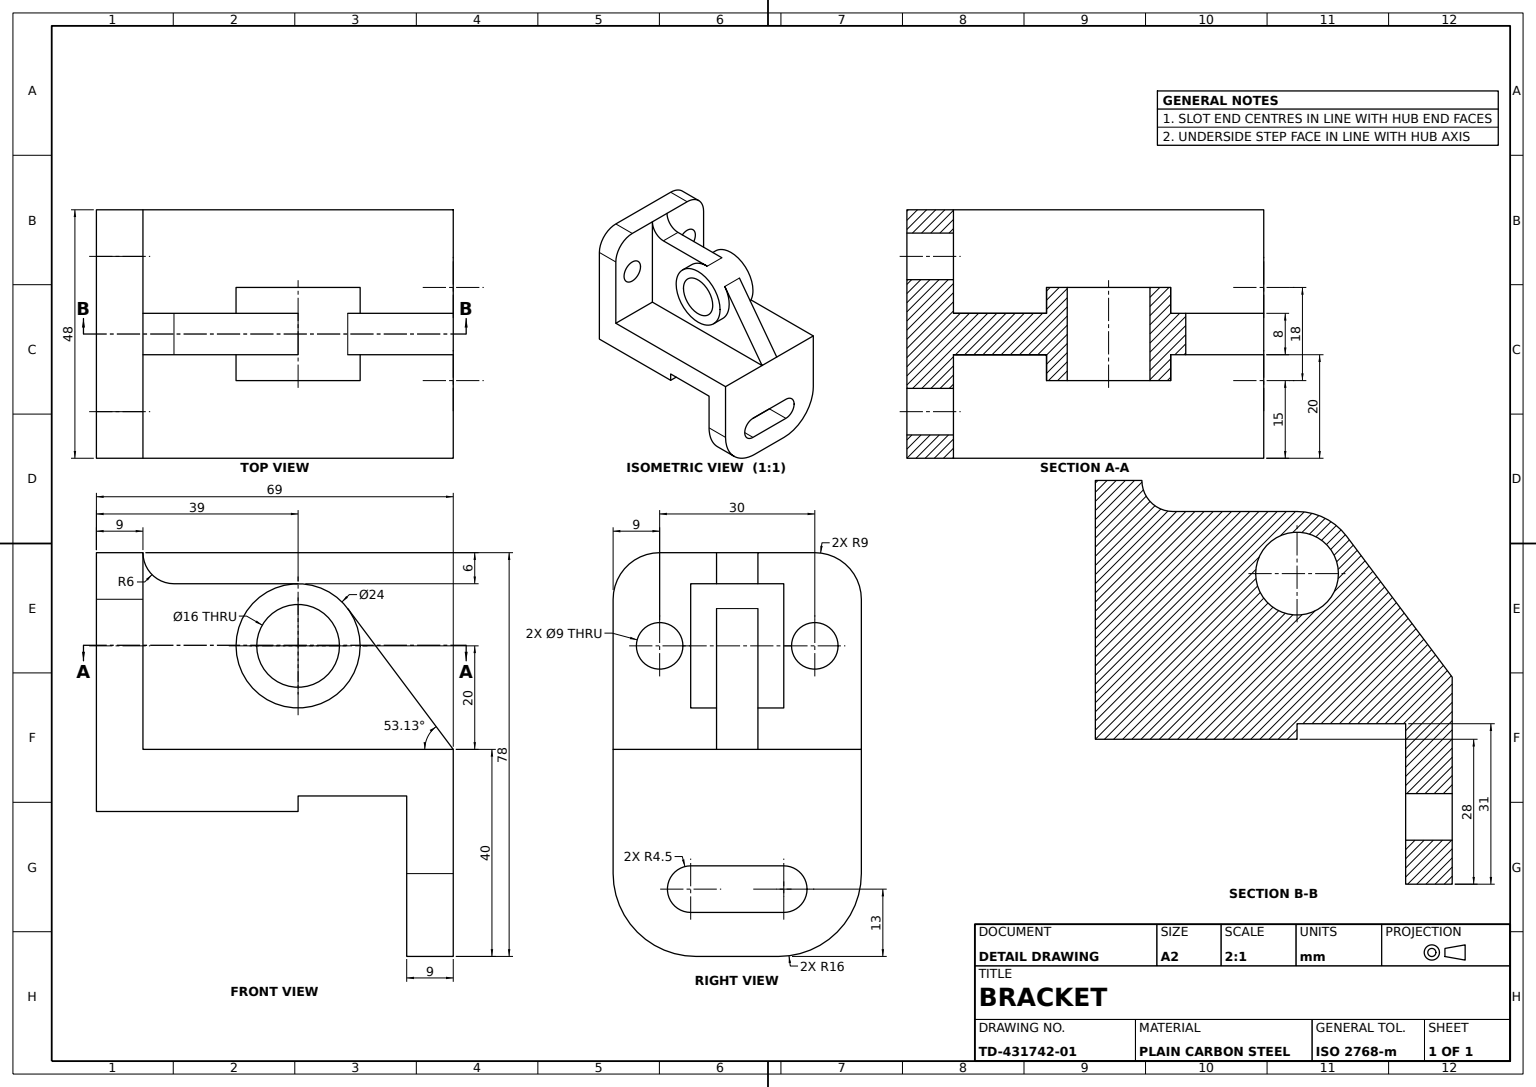
SolidWorks part; units mm, degrees
material "Plain Carbon Steel"
ref_plane "Front Plane" through (0, 0, 0) normal (0, 0, 1) x (1, 0, 0)
ref_plane "Top Plane" through (0, 0, 0) normal (0, 1, 0) x (1, 0, 0)
ref_plane "Right Plane" through (0, 0, 0) normal (1, 0, 0) x (0, 0, -1)
sketch "L Bracket Profile Sketch" plane through (0, 0, 0) normal (0, 0, 1) x (1, 0, 0)
  line L0 (0, 0) -> (39, 0)
  line L1 (39, 0) -> (39, 3)
  line L2 (39, 3) -> (60, 3)
  line L3 (60, 3) -> (60, 0)
  line L4 (60, 0) -> (60, -28)
  line L5 (60, -28) -> (69, -28)
  line L6 (69, -28) -> (69, 12)
  line L7 (69, 12) -> (0, 12)
  line L8 (0, 12) -> (0, 0)
  dimension "D1" = 12
  dimension "D2" = 39
  dimension "D3" = 3
  dimension "D4" = 21
  dimension "D5" = 40
  dimension "D6" = 9
  dimension "D7" = 3
  dimension "D8" = 28
  dimension "D9" = 31
extrude "L Bracket Base" add sketch "L Bracket Profile Sketch" against normal blind 48
fillet "Base Corner Rounds R16" radius 16 2 edges at (64.5, -28, -48) (64.5, -28, 0)
sketch "Slot Sketch" plane through (69, 0, 0) normal (1, 0, 0) x (0, 0, -1)
  line L0 (15, -15) -> (33, -15) construction
  line L1 (15, -10.5) -> (33, -10.5)
  line L2 (15, -19.5) -> (33, -19.5)
  line L3 (32, -28) -> (16, -28) construction
  arc A0 (15, -10.5) -> (15, -19.5) centre (15, -15) ccw
  arc A1 (33, -19.5) -> (33, -10.5) centre (33, -15) ccw
  point P2 (24, -15)
  point P9 (24, -28)
  dimension "D2" = 4.5
  dimension "D1" = 13
  dimension "D3" = 18
  dimension "D4" = 0
extrude "Slot Cut" cut sketch "Slot Sketch" against normal blind 48
sketch "Back Plate Sketch" plane through (0, 0, 0) normal (-1, 0, 0) x (0, 0, 1)
  line L0 (0, 12) -> (0, 50)
  line L1 (0, 50) -> (-48, 50)
  line L2 (-48, 50) -> (-48, 12)
  line L3 (-48, 12) -> (0, 12)
  circle A0 centre (-39, 32) radius 4.5
  circle A1 centre (-9, 32) radius 4.5
  point P11 (-24, 50)
  dimension "D2" = 9
  dimension "D3" = 9
  dimension "D1" = 38
  dimension "D4" = 15
  dimension "D5" = 15
  dimension "D6" = 18
  dimension "D7" = 18
extrude "Back Plate with Mounting Holes 2xØ9" add sketch "Back Plate Sketch" against normal blind 9
ref_plane "Bearing Hub Plane" through (0, 0, -24) normal (0, 0, 1) x (1, 0, 0)
sketch "Bearing Hub Sketch" plane through (0, 0, -24) normal (0, 0, 1) x (1, 0, 0)
  line L1 (69, 12) -> (9, 12) construction
  circle A0 centre (39, 32) radius 12
  circle A1 centre (39, 32) radius 8
  dimension "D1" = 24
  dimension "D2" = 16
  dimension "D3" = 20
  dimension "D4" = 30
extrude "Bearing Hub" add sketch "Bearing Hub Sketch" along normal mid plane 18 separate body
sketch "Support Rib Sketch" plane through (0, 0, -24) normal (0, 0, 1) x (1, 0, 0)
  line L0 (69, 12) -> (48.6, 39.2)
  line L1 (69, 12) -> (9, 12)
  line L2 (9, 12) -> (9, 50)
  line L3 (39, 44) -> (15, 44)
  circle A0 centre (39, 32) radius 12 construction
  arc A1 (9, 50) -> (15, 44) centre (15, 50) ccw
  arc A2 (39, 44) -> (48.6, 39.2) centre (37.9992, 29.9985) cw
  dimension "D1" = 6
  dimension "D2" = 14.0372
extrude "Support Rib" add sketch "Support Rib Sketch" along normal mid plane 8
sketch "Bearing Bore Sketch" plane through (0, 0, -20) normal (0, 0, 1) x (1, 0, 0)
  circle A0 centre (39, 32) radius 8
  dimension "D1" = 16
extrude "Bearing Bore Ø16" cut sketch "Bearing Bore Sketch" against normal through all
fillet "Back Plate Corner Rounds R9" radius 9 2 edges at (4.5, 50, 0) (4.5, 50, -48)
